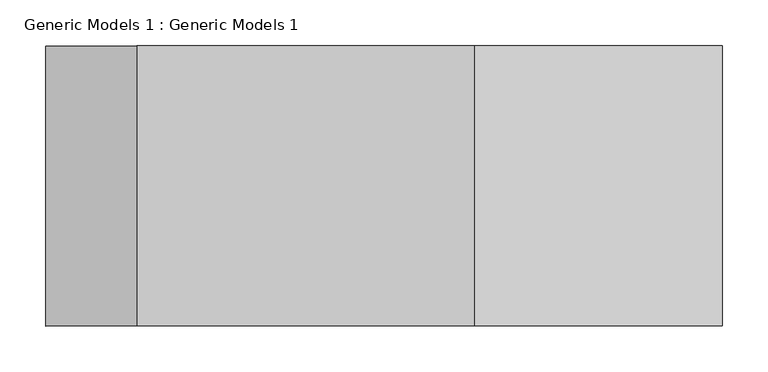
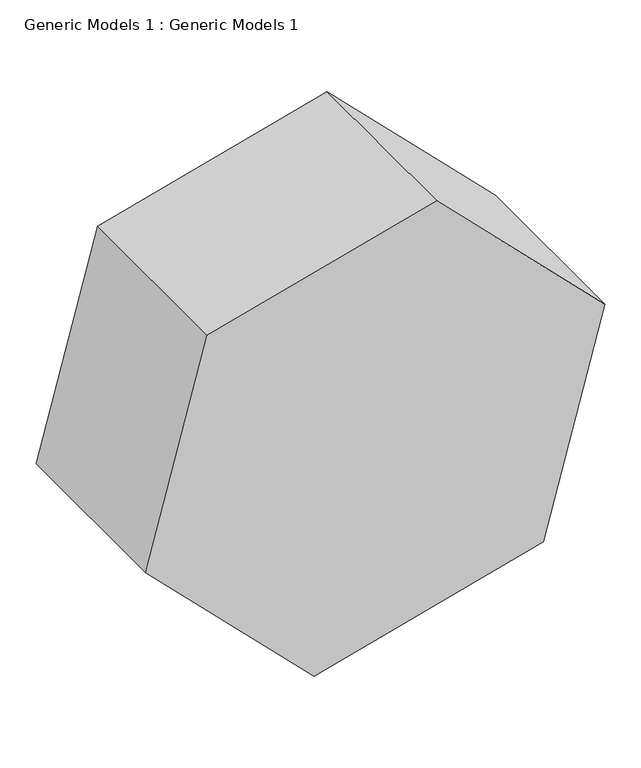
"""IFC4 building model written with IfcOpenShell, lengths in millimetres: proxy geometry, Generic Models 1 : Generic Models 1."""

from ifc_helpers import new_model, si_unit, frame, origin, place, context, project, spatial, polyline, outline, extrude, source, transform, mapped, element, save


def generic_models_1_generic_models_1_b34c57ae(model_context):
    return source(origin(), model_context, "Body", "SweptSolid", [
        extrude(outline(polyline([(708.0393724, -6908.0273199), (977.447056, -7177.4350036), (878.8369998, -7545.4527434), (510.81926, -7644.0627996), (241.4115764, -7374.6551159), (340.0216325, -7006.6373761), (708.0393724, -6908.0273199)])), frame((0.0, -10102.5989753, 0.0), z_axis=(0.0, 1.0, 0.0), x_axis=(0.0, 0.0, 1.0)), (0.0, 0.0, 1.0), 304.8),
    ])


if __name__ == "__main__":
    model = new_model("IFC4")
    model_context = context("Model", 3, world=origin())
    ifc_project = project(units=[si_unit("LENGTHUNIT", "METRE", prefix="MILLI")], contexts=[model_context])
    site = spatial("IfcSite", under=ifc_project)
    building = spatial("IfcBuilding", under=site)
    placement = place(None, origin())
    generic_models_1_generic_models_1_shape = generic_models_1_generic_models_1_b34c57ae(model_context)
    element("IfcBuildingElementProxy", 1, Name="Generic Models 1 : Generic Models 1", ObjectType="Generic Models 1 : Generic Models 1", at=placement, inside=building, context=model_context, shape_type="MappedRepresentation", body=[
        mapped(generic_models_1_generic_models_1_shape, transform((0.0, 0.0, 0.0), x_axis=(1.0, 0.0, 0.0), y_axis=(0.0, 1.0, 0.0), z_axis=(0.0, 0.0, 1.0))),
    ])
    save(model, "model.ifc")
